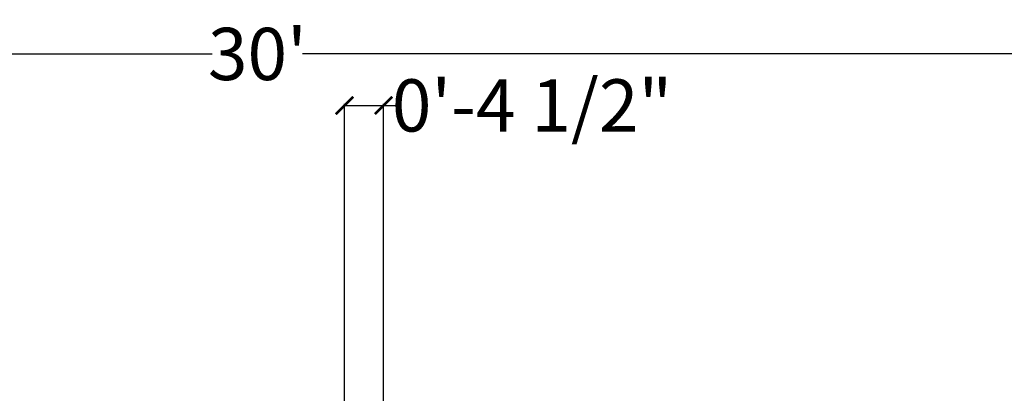
# Model space of a CAD drawing. Units: inches. Extents: x 528 to 2620, y -1066 to 798.
# Tile 18 of 41: x 737 to 850, y 755 to 798. Entities that reach past the tile are written whole.
import ezdxf

# ---------------------------------------------------------------- set-up
doc = ezdxf.new("R2010")
doc.units = ezdxf.units.IN
doc.header["$MEASUREMENT"] = 0
doc.layers.add('A-ANNO-DIMS', color=2, linetype='Continuous', lineweight=18)
doc.styles.get("Standard").update_dxf_attribs({"font": 'arial.ttf'})
doc.dimstyles.get("Standard").update_dxf_attribs({"dimtxt": 6, "dimasz": 2, "dimexe": 0.18, "dimexo": 0.0625, "dimgap": 0.09, "dimtad": 0, "dimtih": 1, "dimtoh": 1, "dimdec": 1, "dimzin": 0, "dimdsep": 46, "dimlunit": 3, "dimtxsty": 'Standard', "dimblk": 'ARCHTICK', "dimcen": 0.09, "dimadec": 0, "dimazin": 0, "dimtfac": 1, "dimtdec": 1, "dimtofl": 0, "dimtmove": 0, "dimatfit": 3, "dimfxl": 1, "dimtolj": 1, "dimtzin": 0, "dimarcsym": 0})

# ---------------------------------------------------------------- blocks, each defined once
blk = doc.blocks.new('_ArchTick')
at = {"color": 0, "linetype": 'ByBlock', "const_width": 0.15}
blk.add_lwpolyline([(-0.5, -0.5), (0.5, 0.5)], dxfattribs=at)
blk = doc.blocks.new('*D11')
at = {"layer": 'A-ANNO-DIMS', "color": 0, "lineweight": -2, "transparency": 16777216}
for p, q in [((584.06, 753.98), (584.06, 794.01)), ((584.06, 793.83), (758.88, 793.83)), ((944.06, 793.83), (769.24, 793.83)), ((944.06, 753.98), (944.06, 794.01))]:
    blk.add_line(p, q, dxfattribs=at)
at = {"layer": 'Defpoints', "color": 0, "transparency": 16777216}
for p in [(944.06, 793.83), (584.06, 753.92), (944.06, 753.92)]:
    blk.add_point(p, dxfattribs=at)
at = {"layer": 'A-ANNO-DIMS', "color": 0, "lineweight": -2, "transparency": 16777216, "xscale": 2, "yscale": 2, "zscale": 2, "rotation": 180}
blk.add_blockref('_ArchTick', (584.06, 793.83), dxfattribs=at)
at = {"layer": 'A-ANNO-DIMS', "color": 0, "lineweight": -2, "transparency": 16777216, "xscale": 2, "yscale": 2, "zscale": 2}
blk.add_blockref('_ArchTick', (944.06, 793.83), dxfattribs=at)
at = {"layer": 'A-ANNO-DIMS', "color": 0, "transparency": 16777216, "insert": (764.06, 793.83), "char_height": 6, "attachment_point": 5}
blk.add_mtext("\\A1;30'", dxfattribs=at)
blk = doc.blocks.new('*D56')
at = {"layer": 'A-ANNO-DIMS', "color": 0, "lineweight": -2, "transparency": 16777216}
for p, q in [((774.06, 709.98), (774.06, 788.1)), ((774.06, 787.92), (778.56, 787.92)), ((778.56, 709.98), (778.56, 788.1)), ((778.56, 787.92), (780.56, 787.92))]:
    blk.add_line(p, q, dxfattribs=at)
at = {"layer": 'Defpoints', "color": 0, "transparency": 16777216}
for p in [(778.56, 787.92), (774.06, 709.92), (778.56, 709.92)]:
    blk.add_point(p, dxfattribs=at)
at = {"layer": 'A-ANNO-DIMS', "color": 0, "lineweight": -2, "transparency": 16777216, "xscale": 2, "yscale": 2, "zscale": 2, "rotation": 180}
blk.add_blockref('_ArchTick', (774.06, 787.92), dxfattribs=at)
at = {"layer": 'A-ANNO-DIMS', "color": 0, "lineweight": -2, "transparency": 16777216, "xscale": 2, "yscale": 2, "zscale": 2}
blk.add_blockref('_ArchTick', (778.56, 787.92), dxfattribs=at)
at = {"layer": 'A-ANNO-DIMS', "color": 0, "transparency": 16777216, "insert": (795.61, 787.92), "char_height": 6, "attachment_point": 5}
blk.add_mtext('\\A1;0\'-4 1/2"', dxfattribs=at)

msp = doc.modelspace()

# ---------------------------------------------------------------- dimensions: what is measured, and where the dimension line sits
at = {"layer": 'A-ANNO-DIMS'}
for base, p1, p2, override, picture, middle in [((944.06, 793.83), (584.06, 753.92), (944.06, 753.92), {"dimclrd": 0, "dimclre": 0, "dimclrt": 0}, '*D11', (764.06, 793.83)), ((778.56, 787.92), (774.06, 709.92), (778.56, 709.92), {"dimdec": 1, "dimlfac": 1, "dimrnd": 0, "dimzin": 1, "dimdsep": 46, "dimlunit": 4, "dimfrac": 2}, '*D56', (795.61, 787.92))]:
    dim = msp.add_linear_dim(base=base, p1=p1, p2=p2, dimstyle='Standard', override=override, dxfattribs=at)
    dim.commit()
    dim.dimension.update_dxf_attribs({"geometry": picture, "text_midpoint": middle})

doc.saveas('drawing.dxf')
